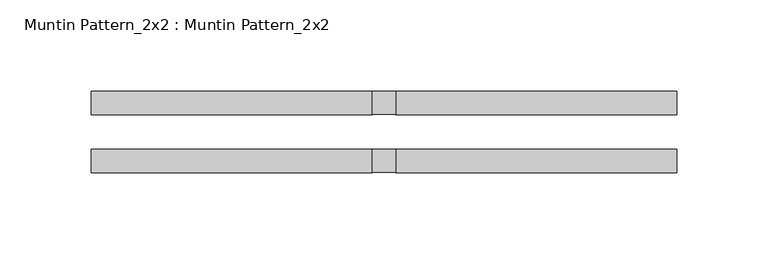
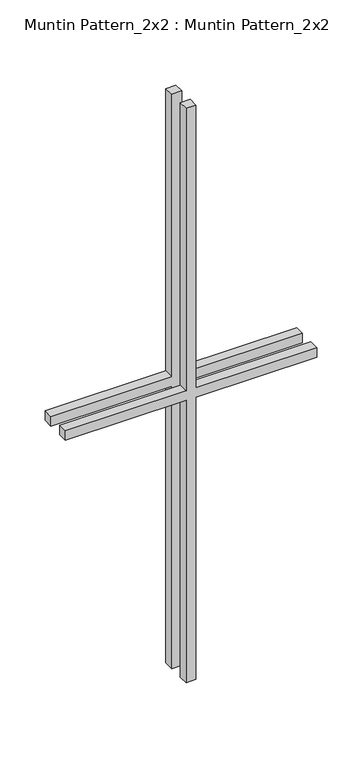
"""IFC4 building model written with IfcOpenShell, lengths in millimetres: proxy geometry, Muntin Pattern_2x2 : Muntin Pattern_2x2."""

from ifc_helpers import new_model, si_unit, frame, origin, place, context, project, spatial, polyline, outline, extrude, source, transform, mapped, element, save


def muntin_pattern_2x2_muntin_pattern_2x2_37b95fb2(model_context):
    return source(origin(), model_context, "Body", "SweptSolid", [
        extrude(outline(polyline([(393.7, -6.35), (393.7, -160.3375), (381.0, -160.3375), (381.0, -6.35), (0.0, -6.35), (0.0, 6.35), (381.0, 6.35), (381.0, 160.3375), (393.7, 160.3375), (393.7, 6.35), (774.7, 6.35), (774.7, -6.35), (393.7, -6.35)])), frame((0.0, -22.225, 0.0), z_axis=(0.0, 1.0, 0.0), x_axis=(0.0, 0.0, 1.0)), (0.0, 0.0, 1.0), 12.7),
        extrude(outline(polyline([(393.7, -6.35), (393.7, -160.3375), (381.0, -160.3375), (381.0, -6.35), (0.0, -6.35), (0.0, 6.35), (381.0, 6.35), (381.0, 160.3375), (393.7, 160.3375), (393.7, 6.35), (774.7, 6.35), (774.7, -6.35), (393.7, -6.35)])), frame((0.0, 9.525, 0.0), z_axis=(0.0, 1.0, 0.0), x_axis=(0.0, 0.0, 1.0)), (0.0, 0.0, 1.0), 12.7),
    ])


if __name__ == "__main__":
    model = new_model("IFC4")
    model_context = context("Model", 3, world=origin())
    ifc_project = project(units=[si_unit("LENGTHUNIT", "METRE", prefix="MILLI")], contexts=[model_context])
    site = spatial("IfcSite", under=ifc_project)
    building = spatial("IfcBuilding", under=site)
    placement = place(None, origin())
    muntin_pattern_2x2_muntin_pattern_2x2_shape = muntin_pattern_2x2_muntin_pattern_2x2_37b95fb2(model_context)
    element("IfcBuildingElementProxy", 1, Name="Muntin Pattern_2x2 : Muntin Pattern_2x2", ObjectType="Muntin Pattern_2x2 : Muntin Pattern_2x2", at=placement, inside=building, context=model_context, shape_type="MappedRepresentation", body=[
        mapped(muntin_pattern_2x2_muntin_pattern_2x2_shape, transform((0.0, 0.0, 0.0), x_axis=(1.0, 0.0, 0.0), y_axis=(0.0, 1.0, 0.0), z_axis=(0.0, 0.0, 1.0))),
    ])
    save(model, "model.ifc")

# Revit data of these elements
# Type "Muntin Pattern_2x2 : Muntin Pattern_2x2"
#   Width [instance default] = 4' - 0"
#   Thickness = 0' - 0 1/2"
#   Height [instance default] = 4' - 0"
#   Distance = 0' - 0 3/4"
#   Interior Material [instance default] = none
#   Exterior Material [instance default] = none
#   Default Elevation = 0
# Element 1 (IfcBuildingElementProxy, "Muntin Pattern_2x2 : Muntin Pattern_2x2")
#   Width = 1' - 0 5/8"
#   Height = 2' - 6 1/2"
#   Interior Material = Wood - Stained
#   Exterior Material = Clad - White
#   Materials on its faces: "Clad - White", "Wood - Stained"
# Materials
#   "Clad - White": class "Wood", colour RGB 242 242 238, transparency 0, Cost = 0
#   "Wood - Stained": class "Wood", colour RGB 224 178 126, transparency 0, Cost = 0
